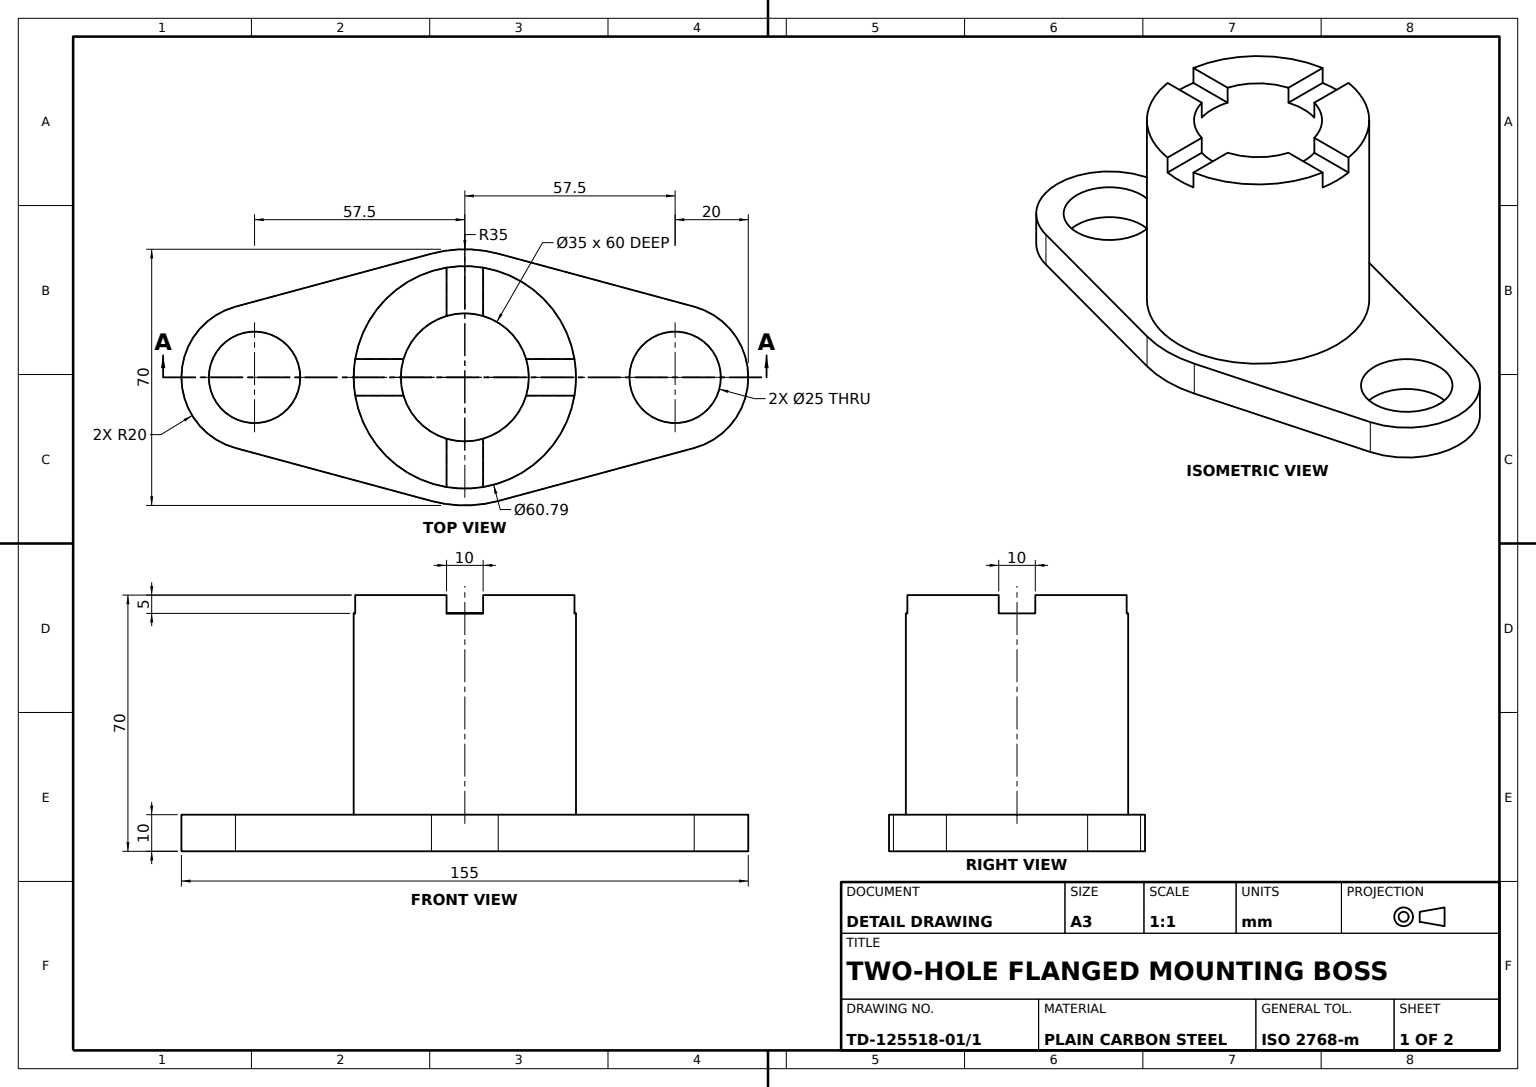
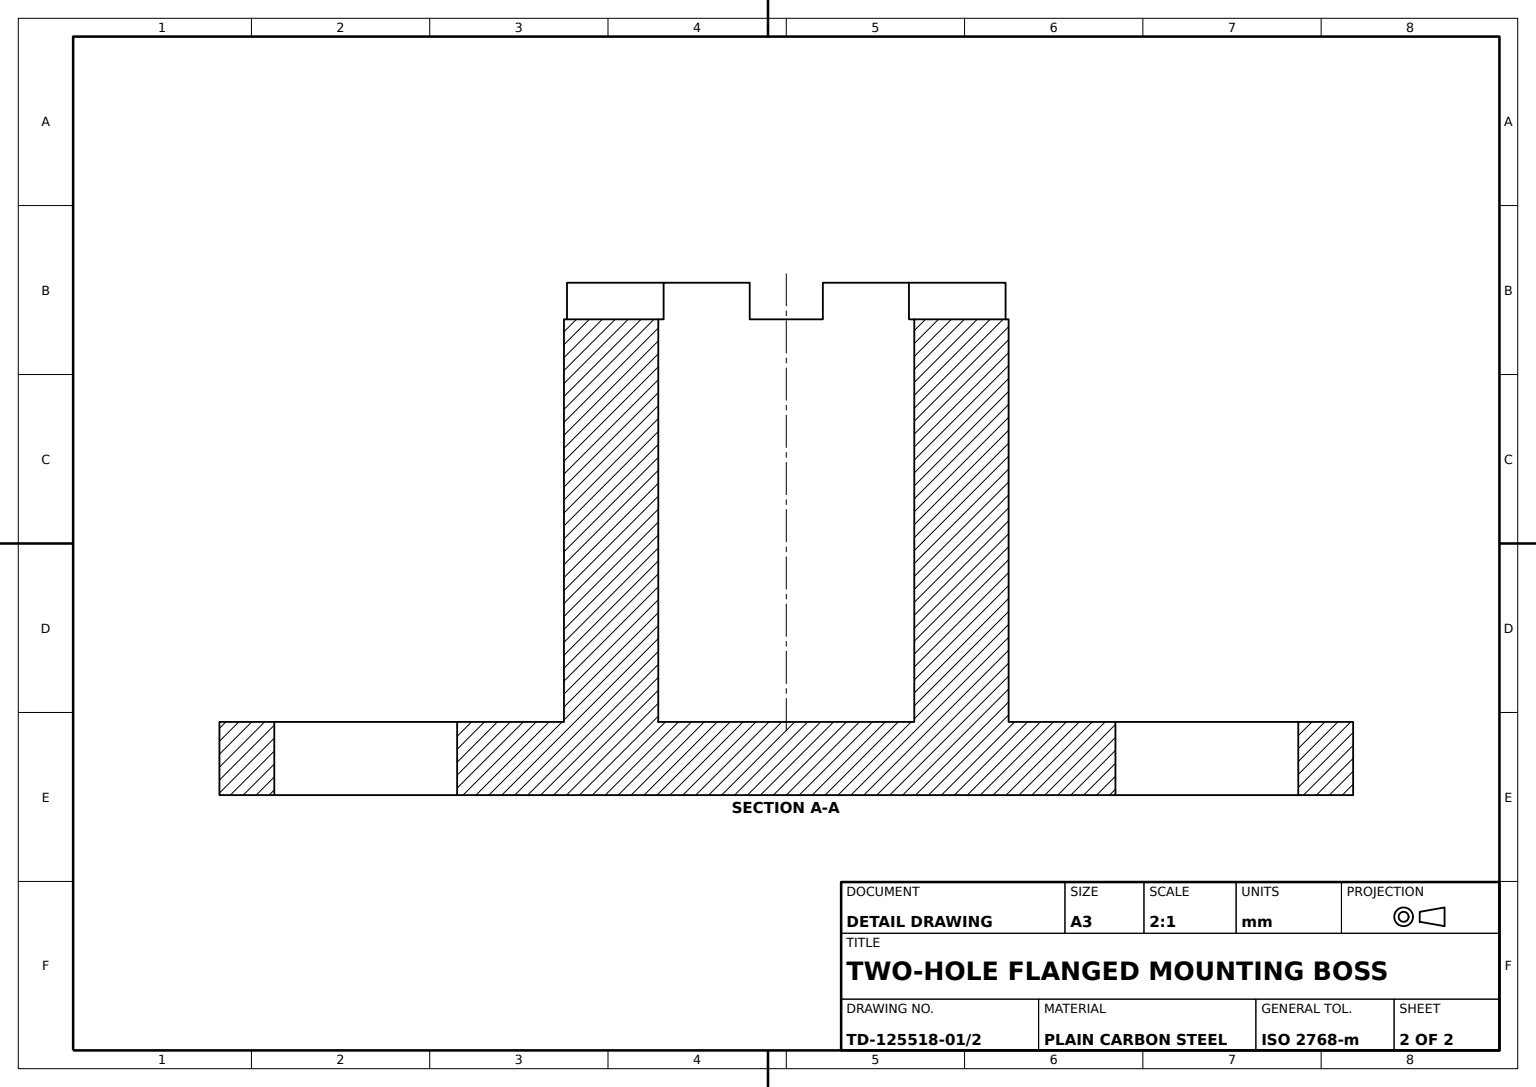
from build123d import *

# Parameters (mm, degrees)
BASE_PLATE_DEPTH             = 10
MOUNTING_HOLES_2X_DEPTH      = 86.622718948
MOUNTING_HOLES_2X_DEPTH_BACK = 86.622718948
MOUNTING_HOLES_PROFILE_R     = 12.5
HUB_PROFILE_R                = 30.395167717
HUB_DEPTH                    = 60
BORE_PROFILE_35_R            = 17.5
BORE_35_DEPTH                = 60
CROSS_SLOTS_4X_DEPTH         = 5


with BuildPart() as part:
    # Base Plate Profile → Base Plate (new body)
    with BuildSketch(Plane(origin=(0, 0, 0), x_dir=(1, 0, 0), z_dir=(0, 1, 0))):
        with BuildLine():
            Line((19.30748114, -62.717391304), (33.788091995, -9.130434783))
            ThreePointArc((33.788091995, -9.130434783), (35, 0), (33.788091995, 9.130434783))
            Line((33.788091995, 9.130434783), (19.30748114, 62.717391304))
            ThreePointArc((19.30748114, 62.717391304), (0, 77.5), (-19.30748114, 62.717391304))
            Line((-19.30748114, 62.717391304), (-33.788091995, 9.130434783))
            ThreePointArc((-33.788091995, 9.130434783), (-35, 0), (-33.788091995, -9.130434783))
            Line((-33.788091995, -9.130434783), (-19.30748114, -62.717391304))
            ThreePointArc((-19.30748114, -62.717391304), (0, -77.5), (19.30748114, -62.717391304))
        make_face()
    extrude(amount=BASE_PLATE_DEPTH)

    # Mounting Holes Profile → Mounting Holes 2x (cut, two sides: drawn at the far end of the back side and taken through both)
    with BuildSketch(Plane(origin=(0, 10, 0), x_dir=(1, 0, 0), z_dir=(0, 1, 0)).offset(-MOUNTING_HOLES_2X_DEPTH_BACK)):
        with Locations(Location((0, 57.5, 0), (0, 0, 270))):
            Circle(MOUNTING_HOLES_PROFILE_R)
        with Locations(Location((0, -57.5, 0), (0, 0, 270))):
            Circle(MOUNTING_HOLES_PROFILE_R)
    extrude(amount=MOUNTING_HOLES_2X_DEPTH + MOUNTING_HOLES_2X_DEPTH_BACK, mode=Mode.SUBTRACT)

    # Hub Profile → Hub (add)
    with BuildSketch(Plane(origin=(0, 10, 0), x_dir=(1, 0, 0), z_dir=(0, 1, 0))):
        with Locations(Location((0, 0, 0), (0, 0, 270))):
            Circle(HUB_PROFILE_R)
    extrude(amount=HUB_DEPTH)

    # Bore Profile Ø35 → Bore Ø35 (cut)
    with BuildSketch(Plane(origin=(0, 70, 0), x_dir=(1, 0, 0), z_dir=(0, 1, 0))):
        with Locations(Location((0, 0, 0), (0, 0, 270))):
            Circle(BORE_PROFILE_35_R)
    extrude(amount=-BORE_35_DEPTH, mode=Mode.SUBTRACT)

    # Cross Slots Profile → Cross Slots 4x (cut)
    with BuildSketch(Plane(origin=(0, 70, 0), x_dir=(1, 0, 0), z_dir=(0, 1, 0))):
        with BuildLine():
            Line((-16.770509831, -5), (-29.981097721, -5))
            ThreePointArc((-29.981097721, -5), (-30.395167717, 0), (-29.981097721, 5))
            Line((-29.981097721, 5), (-16.770509831, 5))
            ThreePointArc((-16.770509831, 5), (-17.5, 0), (-16.770509831, -5))
        make_face()
        with BuildLine():
            Line((-5, -16.770509831), (-5, -29.981097721))
            ThreePointArc((-5, -29.981097721), (0, -30.395167717), (5, -29.981097721))
            Line((5, -29.981097721), (5, -16.770509831))
            ThreePointArc((5, -16.770509831), (0, -17.5), (-5, -16.770509831))
        make_face()
        with BuildLine():
            Line((-5, 16.770509831), (-5, 29.981097721))
            ThreePointArc((-5, 29.981097721), (0, 30.395167717), (5, 29.981097721))
            Line((5, 29.981097721), (5, 16.770509831))
            ThreePointArc((5, 16.770509831), (0, 17.5), (-5, 16.770509831))
        make_face()
        with BuildLine():
            Line((16.770509831, 5), (29.981097721, 5))
            ThreePointArc((29.981097721, 5), (30.395167717, 0), (29.981097721, -5))
            Line((29.981097721, -5), (16.770509831, -5))
            ThreePointArc((16.770509831, -5), (17.5, 0), (16.770509831, 5))
        make_face()
    extrude(amount=-CROSS_SLOTS_4X_DEPTH, mode=Mode.SUBTRACT)


solid = part.part
